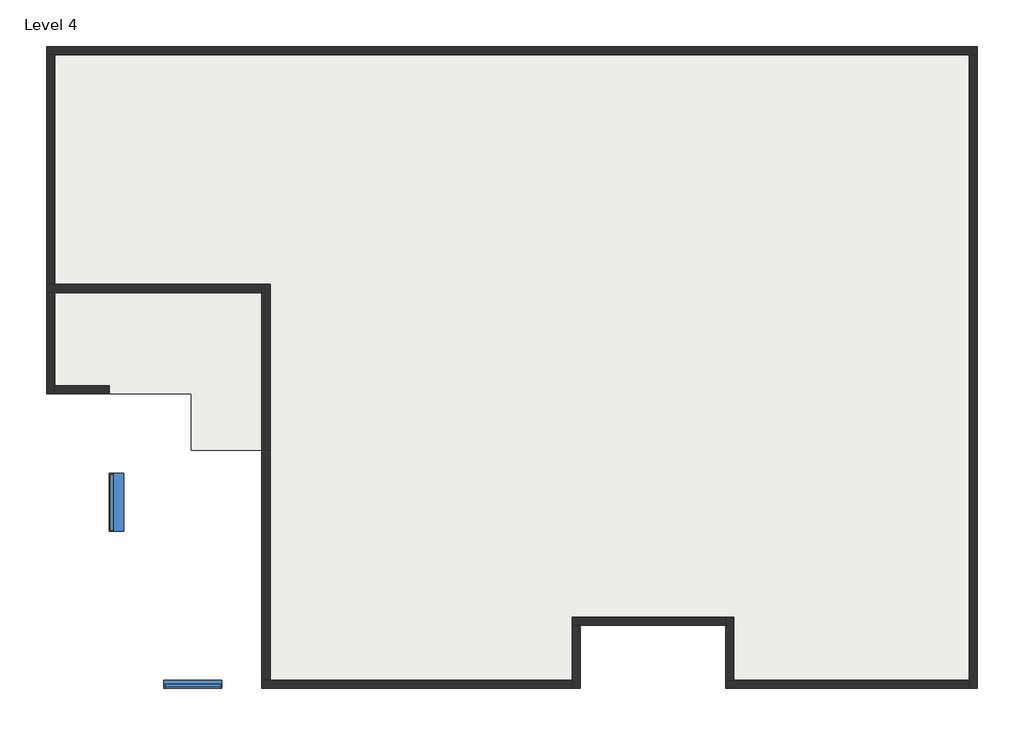
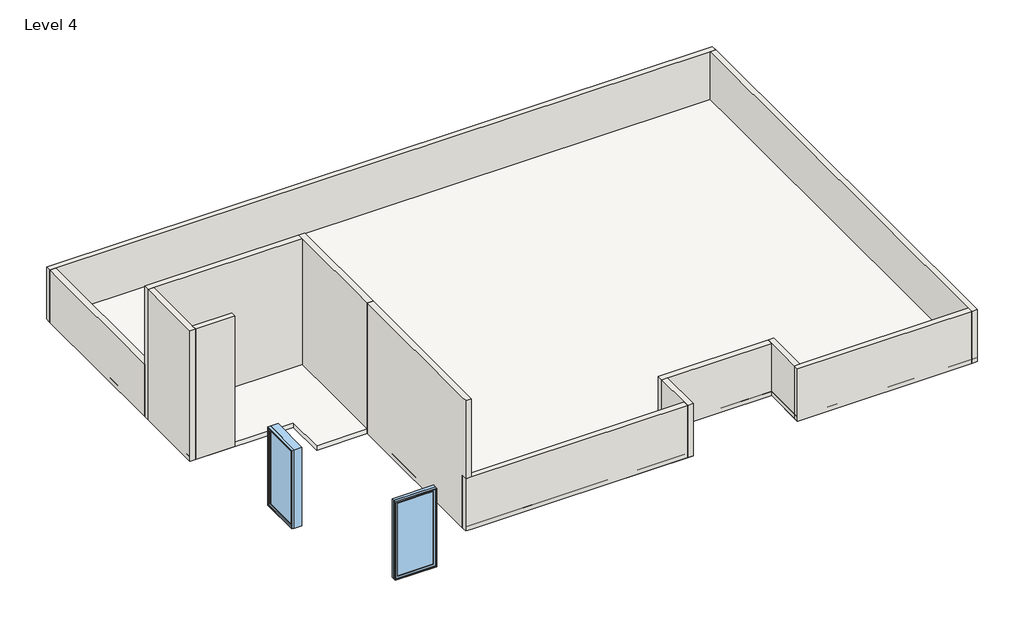
# One storey: 13 walls, 2 windows, 1 roof.
"""IFC4 building model written with IfcOpenShell, lengths in millimetres."""

from ifc_helpers import new_model, si_unit, frame, origin, place, context, project, spatial, polyline, outline, extrude, faceted_brep, transform, mapped, element, save
from components import window_7da3115e, window_c796fc87

model = new_model("IFC4")

# Units and contexts
model_context = context("Model", 3, world=origin())
ifc_project = project(units=[si_unit("LENGTHUNIT", "METRE", prefix="MILLI")], contexts=[model_context])

# Site, building, storey
site = spatial("IfcSite", under=ifc_project)
building = spatial("IfcBuilding", under=site)
storey = spatial("IfcBuildingStorey", under=building, Name="Level 4", Elevation=9144.0)

# Roof
placement = place(None, origin())
element("IfcRoof", 1, ObjectType="Generic - 4\"", at=placement, inside=storey, context=model_context, shape_type="SweptSolid", body=[
    extrude(outline(polyline([(3374.2605242, 2639.8495492), (-600.8394758, 2639.8495492), (-600.8394758, 3630.4495492), (-2899.5394758, 3630.4495492), (-2899.5394758, 2639.8495492), (-7928.7394758, 2639.8495492), (-7928.7394758, 6399.0495492), (-9046.3394758, 6399.0495492), (-9046.3394758, 7288.0495492), (-11332.3394758, 7288.0495492), (-11332.3394758, 12774.4495492), (3374.2605242, 12774.4495492), (3374.2605242, 2639.8495492)])), frame((0.0, 0.0, 9144.0), z_axis=(0.0, 0.0, 1.0), x_axis=(1.0, 0.0, 0.0)), (0.0, 0.0, 1.0), 101.6),
])

# Walls
element("IfcWall", 2, ObjectType="Generic - 5\"", at=placement, inside=storey, context=model_context, shape_type="Brep", body=[
    faceted_brep([(-11332.3394758, 12647.4495492, 9144.0), (-11205.3394758, 12647.4495492, 9144.0), (3247.2605242, 12647.4495492, 9144.0), (3374.2605242, 12647.4495492, 9144.0), (3374.2605242, 12647.4495492, 10363.2), (3247.2605242, 12647.4495492, 10363.2), (-11205.3394758, 12647.4495492, 10363.2), (-11332.3394758, 12647.4495492, 10363.2), (-11332.3394758, 12774.4495492, 9144.0), (-11332.3394758, 12774.4495492, 10363.2), (3374.2605242, 12774.4495492, 10363.2), (3374.2605242, 12774.4495492, 9144.0)], [[[0, 1, 2, 3, 4, 5, 6, 7]], [[8, 9, 10, 11]], [[3, 2, 1, 0, 8, 11]], [[7, 6, 5, 4, 10, 9]], [[4, 3, 11, 10]], [[0, 7, 9, 8]]]),
])
element("IfcWall", 3, ObjectType="Generic - 5\"", at=placement, inside=storey, context=model_context, shape_type="Brep", body=[
    faceted_brep([(3247.2605242, 12647.4495492, 9144.0), (3247.2605242, 2766.8495492, 9144.0), (3247.2605242, 2639.8495492, 9144.0), (3247.2605242, 2639.8495492, 10363.2), (3247.2605242, 2766.8495492, 10363.2), (3247.2605242, 12647.4495492, 10363.2), (3374.2605242, 12647.4495492, 9144.0), (3374.2605242, 12647.4495492, 10363.2), (3374.2605242, 2639.8495492, 10363.2), (3374.2605242, 2639.8495492, 9144.0)], [[[0, 1, 2, 3, 4, 5]], [[6, 7, 8, 9]], [[2, 1, 0, 6, 9]], [[5, 4, 3, 8, 7]], [[0, 5, 7, 6]], [[3, 2, 9, 8]]]),
])
element("IfcWall", 4, ObjectType="Generic - 5\"", at=placement, inside=storey, context=model_context, shape_type="Brep", body=[
    faceted_brep([(3247.2605242, 2766.8495492, 9144.0), (-473.8394758, 2766.8495492, 9144.0), (-600.8394758, 2766.8495492, 9144.0), (-600.8394758, 2766.8495492, 10363.2), (-473.8394758, 2766.8495492, 10363.2), (3247.2605242, 2766.8495492, 10363.2), (3247.2605242, 2639.8495492, 9144.0), (3247.2605242, 2639.8495492, 10363.2), (-600.8394758, 2639.8495492, 10363.2), (-600.8394758, 2639.8495492, 9144.0)], [[[0, 1, 2, 3, 4, 5]], [[6, 7, 8, 9]], [[2, 1, 0, 6, 9]], [[5, 4, 3, 8, 7]], [[0, 5, 7, 6]], [[3, 2, 9, 8]]]),
])
element("IfcWall", 5, ObjectType="Generic - 5\"", at=placement, inside=storey, context=model_context, shape_type="Brep", body=[
    faceted_brep([(-473.8394758, 2766.8495492, 9144.0), (-473.8394758, 3757.4495492, 9144.0), (-473.8394758, 3757.4495492, 10363.2), (-473.8394758, 2766.8495492, 10363.2), (-600.8394758, 2766.8495492, 9144.0), (-600.8394758, 2766.8495492, 10363.2), (-600.8394758, 3630.4495492, 10363.2), (-600.8394758, 3757.4495492, 10363.2), (-600.8394758, 3757.4495492, 9144.0), (-600.8394758, 3630.4495492, 9144.0)], [[[0, 1, 2, 3]], [[4, 5, 6, 7, 8, 9]], [[1, 0, 4, 9, 8]], [[3, 2, 7, 6, 5]], [[0, 3, 5, 4]], [[2, 1, 8, 7]]]),
])
element("IfcWall", 6, ObjectType="Generic - 5\"", at=placement, inside=storey, context=model_context, shape_type="Brep", body=[
    faceted_brep([(-600.8394758, 3757.4495492, 9144.0), (-3026.5394758, 3757.4495492, 9144.0), (-3026.5394758, 3757.4495492, 10363.2), (-600.8394758, 3757.4495492, 10363.2), (-600.8394758, 3630.4495492, 9144.0), (-600.8394758, 3630.4495492, 10363.2), (-2899.5394758, 3630.4495492, 10363.2), (-3026.5394758, 3630.4495492, 10363.2), (-3026.5394758, 3630.4495492, 9144.0), (-2899.5394758, 3630.4495492, 9144.0)], [[[0, 1, 2, 3]], [[4, 5, 6, 7, 8, 9]], [[1, 0, 4, 9, 8]], [[3, 2, 7, 6, 5]], [[0, 3, 5, 4]], [[2, 1, 8, 7]]]),
])
element("IfcWall", 7, ObjectType="Generic - 5\"", at=placement, inside=storey, context=model_context, shape_type="Brep", body=[
    faceted_brep([(-3026.5394758, 3630.4495492, 9144.0), (-3026.5394758, 2766.8495492, 9144.0), (-3026.5394758, 2639.8495492, 9144.0), (-3026.5394758, 2639.8495492, 10363.2), (-3026.5394758, 2766.8495492, 10363.2), (-3026.5394758, 3630.4495492, 10363.2), (-2899.5394758, 3630.4495492, 9144.0), (-2899.5394758, 3630.4495492, 10363.2), (-2899.5394758, 2639.8495492, 10363.2), (-2899.5394758, 2639.8495492, 9144.0)], [[[0, 1, 2, 3, 4, 5]], [[6, 7, 8, 9]], [[2, 1, 0, 6, 9]], [[5, 4, 3, 8, 7]], [[0, 5, 7, 6]], [[3, 2, 9, 8]]]),
])
element("IfcWall", 8, ObjectType="Generic - 5\"", at=placement, inside=storey, context=model_context, shape_type="Brep", body=[
    faceted_brep([(-3026.5394758, 2766.8495492, 9144.0), (-7801.7394758, 2766.8495492, 9144.0), (-7928.7394758, 2766.8495492, 9144.0), (-7928.7394758, 2766.8495492, 10363.2), (-7801.7394758, 2766.8495492, 10363.2), (-3026.5394758, 2766.8495492, 10363.2), (-3026.5394758, 2639.8495492, 9144.0), (-3026.5394758, 2639.8495492, 10363.2), (-7801.7394758, 2639.8495492, 10363.2), (-7928.7394758, 2639.8495492, 10363.2), (-7928.7394758, 2639.8495492, 9144.0), (-7801.7394758, 2639.8495492, 9144.0)], [[[0, 1, 2, 3, 4, 5]], [[6, 7, 8, 9, 10, 11]], [[2, 1, 0, 6, 11, 10]], [[5, 4, 3, 9, 8, 7]], [[0, 5, 7, 6]], [[3, 2, 10, 9]]]),
])
element("IfcWall", 9, ObjectType="Generic - 5\"", at=placement, inside=storey, context=model_context, shape_type="Brep", body=[
    faceted_brep([(-7801.7394758, 2766.8495492, 9144.0), (-7801.7394758, 6399.0495492, 9144.0), (-7801.7394758, 6399.0495492, 12192.0), (-7801.7394758, 2639.8495492, 12192.0), (-7801.7394758, 2639.8495492, 10363.2), (-7801.7394758, 2766.8495492, 10363.2), (-7928.7394758, 2766.8495492, 9144.0), (-7928.7394758, 2766.8495492, 10363.2), (-7928.7394758, 2639.8495492, 10363.2), (-7928.7394758, 2639.8495492, 12192.0), (-7928.7394758, 2766.8495492, 12192.0), (-7928.7394758, 6399.0495492, 12192.0), (-7928.7394758, 6399.0495492, 9144.0)], [[[0, 1, 2, 3, 4, 5]], [[6, 7, 8, 9, 10, 11, 12]], [[1, 0, 6, 12]], [[2, 1, 12, 11]], [[3, 2, 11, 10, 9]], [[4, 8, 7, 5]], [[0, 5, 7, 6]], [[4, 3, 9, 8]]]),
])
element("IfcWall", 10, ObjectType="Generic - 5\"", at=placement, inside=storey, context=model_context, shape_type="Brep", body=[
    faceted_brep([(-7928.7394758, 9015.2495492, 9144.0), (-11205.3394758, 9015.2495492, 9144.0), (-11332.3394758, 9015.2495492, 9144.0), (-11332.3394758, 9015.2495492, 10363.2), (-11332.3394758, 9015.2495492, 12192.0), (-7928.7394758, 9015.2495492, 12192.0), (-7928.7394758, 8888.2495492, 9144.0), (-7928.7394758, 8888.2495492, 12192.0), (-11205.3394758, 8888.2495492, 12192.0), (-11332.3394758, 8888.2495492, 12192.0), (-11332.3394758, 8888.2495492, 9144.0), (-11205.3394758, 8888.2495492, 9144.0)], [[[0, 1, 2, 3, 4, 5]], [[6, 7, 8, 9, 10, 11]], [[2, 1, 0, 6, 11, 10]], [[5, 4, 9, 8, 7]], [[0, 5, 7, 6]], [[2, 10, 9, 4, 3]]]),
])
element("IfcWall", 11, ObjectType="Generic - 5\"", at=placement, inside=storey, context=model_context, shape_type="SweptSolid", body=[
    extrude(outline(polyline([(-11205.3394758, 12647.4495492), (-11205.3394758, 9015.2495492), (-11332.3394758, 9015.2495492), (-11332.3394758, 12647.4495492), (-11205.3394758, 12647.4495492)])), frame((0.0, 0.0, 9144.0), z_axis=(0.0, 0.0, 1.0), x_axis=(1.0, 0.0, 0.0)), (0.0, 0.0, 1.0), 1219.2),
])
element("IfcWall", 12, ObjectType="Generic - 5\"", at=placement, inside=storey, context=model_context, shape_type="Brep", body=[
    faceted_brep([(-11332.3394758, 8888.2495492, 9144.0), (-11332.3394758, 7288.0495492, 9144.0), (-11332.3394758, 7288.0495492, 12192.0), (-11332.3394758, 8888.2495492, 12192.0), (-11205.3394758, 8888.2495492, 9144.0), (-11205.3394758, 8888.2495492, 12192.0), (-11205.3394758, 7415.0495492, 12192.0), (-11205.3394758, 7288.0495492, 12192.0), (-11205.3394758, 7288.0495492, 9144.0), (-11205.3394758, 7415.0495492, 9144.0)], [[[0, 1, 2, 3]], [[4, 5, 6, 7, 8, 9]], [[1, 0, 4, 9, 8]], [[3, 2, 7, 6, 5]], [[0, 3, 5, 4]], [[2, 1, 8, 7]]]),
])
element("IfcWall", 13, ObjectType="Generic - 5\"", at=placement, inside=storey, context=model_context, shape_type="Brep", body=[
    faceted_brep([(-11205.3394758, 7288.0495492, 9144.0), (-10341.7394758, 7288.0495492, 9144.0), (-10341.7394758, 7288.0495492, 12192.0), (-11205.3394758, 7288.0495492, 12192.0), (-11205.3394758, 7415.0495492, 9144.0), (-11205.3394758, 7415.0495492, 12192.0), (-10341.7394758, 7415.0495492, 12192.0), (-10341.7394758, 7415.0495492, 9144.0), (-10341.7394758, 7351.5495492, 9144.0)], [[[0, 1, 2, 3]], [[4, 5, 6, 7]], [[1, 0, 4, 7, 8]], [[3, 2, 6, 5]], [[0, 3, 5, 4]], [[2, 1, 8, 7, 6]]]),
])
element("IfcWall", 14, ObjectType="Generic - 5\"", at=placement, inside=storey, context=model_context, shape_type="Brep", body=[
    faceted_brep([(-7801.7394758, 6399.0495492, 9144.0), (-7801.7394758, 9015.2495492, 9144.0), (-7801.7394758, 9015.2495492, 12192.0), (-7801.7394758, 6399.0495492, 12192.0), (-7928.7394758, 6399.0495492, 9144.0), (-7928.7394758, 6399.0495492, 12192.0), (-7928.7394758, 8888.2495492, 12192.0), (-7928.7394758, 9015.2495492, 12192.0), (-7928.7394758, 9015.2495492, 9144.0), (-7928.7394758, 8888.2495492, 9144.0)], [[[0, 1, 2, 3]], [[4, 5, 6, 7, 8, 9]], [[1, 0, 4, 9, 8]], [[3, 2, 7, 6, 5]], [[0, 3, 5, 4]], [[2, 1, 8, 7]]]),
])

# Windows
window_shape = window_7da3115e(model_context)
element("IfcWindow", 15, ObjectType="Fixed : 36\" x 72\"", at=placement, inside=storey, context=model_context, shape_type="MappedRepresentation", body=[
    mapped(window_shape, transform((-9059.0394758, 2703.3495492, 8229.6), x_axis=(-1.0, 0.0, 0.0), y_axis=(0.0, -1.0, 0.0), z_axis=(0.0, 0.0, 1.0))),
])
window_2_shape = window_c796fc87(model_context)
element("IfcWindow", 16, ObjectType="Fixed : 36\" x 72\"", at=placement, inside=storey, context=model_context, shape_type="MappedRepresentation", body=[
    mapped(window_2_shape, transform((-10227.4394758, 5611.6495492, 8229.6), x_axis=(0.0, 1.0, 0.0), y_axis=(-1.0, 0.0, 0.0), z_axis=(0.0, 0.0, 1.0))),
])

save(model, "model.ifc")

# Revit data of these elements
# Type "Generic - 4\""
#   Assembly Code = "B1020"
#   Layers, outside or top first: 0' - 4" "01 colour 1" (function 1)
# Type "Generic - 5\""
#   Assembly Code = "B2010"
#   Layers, outside or top first: 0' - 5" no material (function 1)
# Type "Fixed : 36\" x 72\""
#   Type Mark = "9"
#   Assembly Code = "B2020100"
#   Height = 6' - 0"
#   Default Sill Height = 1' - 0"
#   Width = 3' - 0"
#   Window Inset = 0' - 0 3/4"
#   Glass Pane Material = Glass
#   Sash Material = Sash
#   Wall Closure = (empty or 0)
# Element 1 (IfcRoof, "Generic - 4\"")
#   built-in parameter 1001705 = 30.3333 (stored number, unit not read)
#   built-in parameter 1001710 = 33615
#   Phase Created = New Construction
#   Materials on its faces: "01 colour 1"
# Element 2 (IfcWall, "Generic - 5\"")
#   Top Offset = 0' - 0"
#   Base Offset = 0' - 0"
#   Unconnected Height = 4' - 0"
#   wall height = 4' - 0"
#   Phase Created = New Construction
#   Base Constraint = Level 4
#   Materials on its faces: "Default Wall", "02 white", "01 colour 1(1)"
# Element 3 (IfcWall, "Generic - 5\"")
#   Top Offset = 0' - 0"
#   Base Offset = 0' - 0"
#   Unconnected Height = 4' - 0"
#   wall height = 4' - 0"
#   Phase Created = New Construction
#   Base Constraint = Level 4
#   Materials on its faces: "Default Wall", "01 colour 1(1)", "02 white", "01 colour 1"
# Elements 4, 5, 6, 7, 8 (IfcWall, "Generic - 5\"")
#   Top Offset = 0' - 0"
#   Base Offset = 0' - 0"
#   Unconnected Height = 4' - 0"
#   wall height = 4' - 0"
#   Phase Created = New Construction
#   Base Constraint = Level 4
#   Materials on its faces: "Default Wall", "01 colour 1"
# Elements 9, 12, 13 (IfcWall, "Generic - 5\"")
#   Top Offset = 0' - 0"
#   Base Offset = 0' - 0"
#   Unconnected Height = 10' - 0"
#   wall height = 10' - 0"
#   Phase Created = New Construction
#   Base Constraint = Level 4
#   Materials on its faces: "Default Wall", "01 colour 1"
# Elements 10, 14 (IfcWall, "Generic - 5\"")
#   Top Offset = 0' - 0"
#   Base Offset = 0' - 0"
#   Unconnected Height = 10' - 0"
#   wall height = 10' - 0"
#   Phase Created = New Construction
#   Base Constraint = Level 4
#   Materials on its faces: "Default Wall"
# Element 11 (IfcWall, "Generic - 5\"")
#   Top Offset = 0' - 0"
#   Base Offset = 0' - 0"
#   Unconnected Height = 4' - 0"
#   wall height = 4' - 0"
#   Phase Created = New Construction
#   Base Constraint = Level 4
#   Materials on its faces: "Default Wall"
# Element 15 (IfcWindow, "Fixed : 36\" x 72\"")
#   Mark = "6"
#   Phase Created = New Construction
#   Materials on its faces: "Sash", "Glass"
# Element 16 (IfcWindow, "Fixed : 36\" x 72\"")
#   Mark = "20"
#   Phase Created = New Construction
#   Materials on its faces: "Sash", "Glass"
# Materials
#   "01 colour 1": class "Generic", colour RGB 120 120 120, transparency 0, Cost = 0
#   "Glass": class "Glass", colour RGB 218 227 224, transparency 0.85, Description = "Soda Lime Glass", Cost = 0
#   "Sash": class "Wood", colour RGB 136 99 55, transparency 0
#   "Default Wall": colour RGB 80 80 80, transparency 0
#   "02 white": class "Generic", colour RGB 120 120 120, transparency 0, Cost = 0
#   "01 colour 1(1)": class "Generic", colour RGB 120 120 120, transparency 0, Cost = 0
